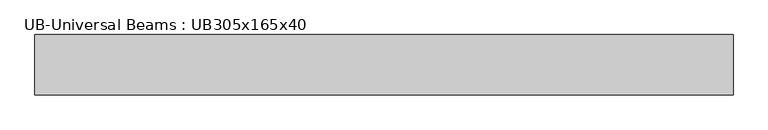
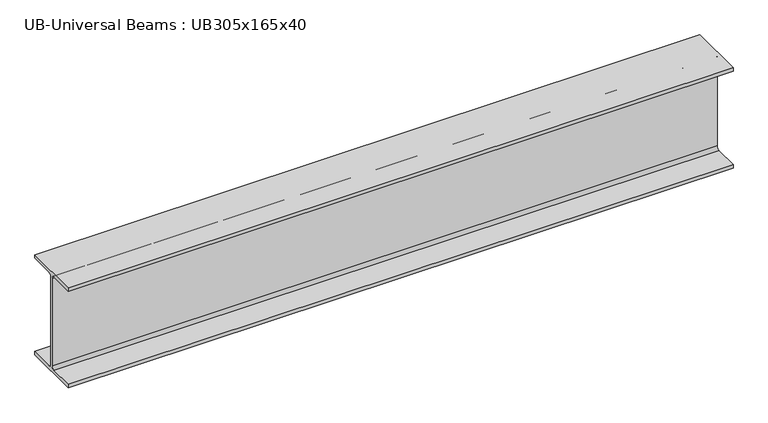
"""IFC4 building model written with IfcOpenShell, lengths in millimetres: beam geometry, UB-Universal Beams : UB305x165x40."""

from ifc_helpers import new_model, si_unit, point, frame, frame_2d, origin, place, context, project, spatial, polyline, circle_curve, trimmed, segment, composite_curve, outline, extrude, source, transform, mapped, element, save


def ub_universal_beams_ub305x165x40_94bf3abd(model_context):
    return source(origin(), model_context, "Body", "SweptSolid", [
        extrude(outline(composite_curve([segment(polyline([(82.5, -141.5), (82.5, -151.7), (-82.5, -151.7), (-82.5, -141.5), (-11.9, -141.5)]), True, "CONTINUOUS"), segment(trimmed(circle_curve(frame_2d((-11.9, -132.6)), 8.9), [point((-11.9, -141.5))], [point((-3.0, -132.6))], True, "CARTESIAN"), True, "CONTINUOUS"), segment(polyline([(-3.0, -132.6), (-3.0, 132.6)]), True, "CONTINUOUS"), segment(trimmed(circle_curve(frame_2d((-11.9, 132.6)), 8.9), [point((-3.0, 132.6))], [point((-11.9, 141.5))], True, "CARTESIAN"), True, "CONTINUOUS"), segment(polyline([(-11.9, 141.5), (-82.5, 141.5), (-82.5, 151.7), (82.5, 151.7), (82.5, 141.5), (11.9, 141.5)]), True, "CONTINUOUS"), segment(trimmed(circle_curve(frame_2d((11.9, 132.6)), 8.9), [point((11.9, 141.5))], [point((3.0, 132.6))], True, "CARTESIAN"), True, "CONTINUOUS"), segment(polyline([(3.0, 132.6), (3.0, -132.6)]), True, "CONTINUOUS"), segment(trimmed(circle_curve(frame_2d((11.9, -132.6)), 8.9), [point((3.0, -132.6))], [point((11.9, -141.5))], True, "CARTESIAN"), True, "CONTINUOUS"), segment(polyline([(11.9, -141.5), (82.5, -141.5)]), True, "CONTINUOUS")], self_intersect=False)), frame((-835.05, 0.0, 0.0), z_axis=(1.0, 0.0, 0.0), x_axis=(0.0, 1.0, 0.0)), (0.0, 0.0, 1.0), 1905.0),
    ])


if __name__ == "__main__":
    model = new_model("IFC4")
    model_context = context("Model", 3, world=origin())
    ifc_project = project(units=[si_unit("LENGTHUNIT", "METRE", prefix="MILLI")], contexts=[model_context])
    site = spatial("IfcSite", under=ifc_project)
    building = spatial("IfcBuilding", under=site)
    placement = place(None, origin())
    ub_universal_beams_ub305x165x40_shape = ub_universal_beams_ub305x165x40_94bf3abd(model_context)
    element("IfcBeam", 1, ObjectType="UB-Universal Beams : UB305x165x40", at=placement, inside=building, context=model_context, shape_type="MappedRepresentation", body=[
        mapped(ub_universal_beams_ub305x165x40_shape, transform((0.0, 0.0, 0.0), x_axis=(1.0, 0.0, 0.0), y_axis=(0.0, 1.0, 0.0), z_axis=(0.0, 0.0, 1.0))),
    ])
    save(model, "model.ifc")

# Revit data of these elements
# Type "UB-Universal Beams : UB305x165x40"
#   Section Name Key = "UB305X165X40"
#   Width = 16.5 cm
#   Web Thickness = 0.6 cm
#   Web Fillet = 0.89 cm
#   Warping Constant = 164000.0 cm⁶
#   Torsional Moment of Inertia = 14.70 cm⁴
#   Section Area = 51.3 cm²
#   Plastic Modulus weak axis = 142.0 cm³
#   Plastic Modulus strong axis = 623.0 cm³
#   Nominal Weight = 40.2999 kgf/m
#   Moment of Inertia weak axis = 764.00 cm⁴
#   Moment of Inertia strong axis = 8503.00 cm⁴
#   Height = 30.34 cm
#   Flange Thickness = 1.02 cm
#   Elastic Modulus weak axis = 92.6 cm³
#   Elastic Modulus strong axis = 560.0 cm³
#   Centroid Vertical = 15.17 cm
#   Centroid Horizontal = 8.25 cm
#   Bolt Spacing = 9.0 cm
#   Length [instance default] = 1500 mm
#   Structural Material [instance default] = Metal - Steel 43-275
#   Type Comments = ""
#   Assembly Code = ""
# Element 1 (IfcBeam, "UB-Universal Beams : UB305x165x40")
#   Materials on its faces: "Metal - Steel 43-275"
# Materials
#   "Metal - Steel 43-275": class "Metal", colour RGB 247 247 247, transparency 0, Cost = 0
